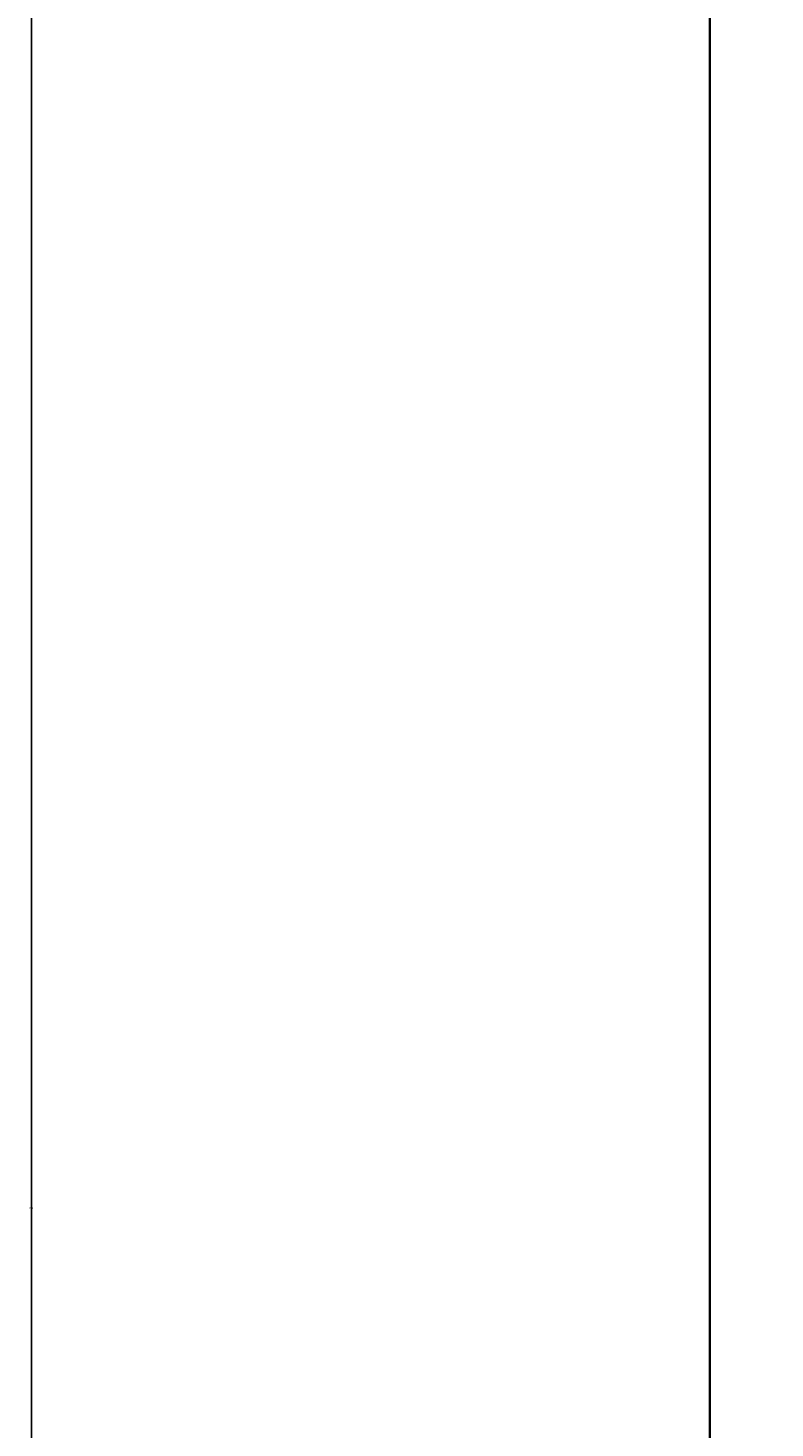
# Model space of a CAD drawing. Units: inches. Extents: x -61 to 1599, y -1316 to 257.
# Tile 96 of 204: x -61 to 22, y -166 to -10. Entities that reach past the tile are written whole.
import ezdxf

# ---------------------------------------------------------------- set-up
doc = ezdxf.new("R2010")
doc.units = ezdxf.units.IN
doc.header["$MEASUREMENT"] = 0
doc.layers.add('A-ANNO-DIMS', color=2, linetype='Continuous', lineweight=18)
doc.layers.add('WALLS', color=4, linetype='Continuous', lineweight=35)
doc.styles.get("Standard").update_dxf_attribs({"font": 'arial.ttf'})
doc.dimstyles.get("Standard").update_dxf_attribs({"dimtxt": 0.18, "dimasz": 0.18, "dimexe": 0.18, "dimexo": 0.0625, "dimgap": 0.09, "dimtad": 0, "dimtih": 1, "dimtoh": 1, "dimdec": 0, "dimzin": 0, "dimdsep": 46, "dimlunit": 3, "dimtxsty": 'Standard', "dimcen": 0.09, "dimadec": 0, "dimazin": 0, "dimtfac": 1, "dimtdec": 0, "dimtofl": 0, "dimtmove": 0, "dimatfit": 3, "dimfxl": 1, "dimtolj": 1, "dimtzin": 0, "dimarcsym": 0})

# ---------------------------------------------------------------- blocks, each defined once
blk = doc.blocks.new('*D687')
at = {"layer": 'A-ANNO-DIMS', "color": 0, "lineweight": -2, "transparency": 16777216}
for p, q in [((289.42, 181.68), (-61.08, 181.68)), ((-60.9, 181.5), (-60.9, -528.95)), ((-60.9, -1239.76), (-60.9, -529.32)), ((319.64, -1239.94), (-61.08, -1239.94))]:
    blk.add_line(p, q, dxfattribs=at)
at = {"layer": 'A-ANNO-DIMS', "color": 0, "transparency": 16777216}
for points in [[(-60.93, 181.5), (-60.87, 181.5), (-60.9, 181.68)], [(-60.93, -1239.76), (-60.87, -1239.76), (-60.9, -1239.94)]]:
    blk.add_solid(points, dxfattribs=at)
at = {"layer": 'DEFPOINTS', "color": 0, "transparency": 16777216}
for p in [(289.48, 181.68), (-60.9, -1239.94), (319.7, -1239.94)]:
    blk.add_point(p, dxfattribs=at)
at = {"layer": 'A-ANNO-DIMS', "color": 0, "transparency": 16777216, "insert": (-60.9, -529.13), "char_height": 0.18, "attachment_point": 5}
blk.add_mtext('\\A1;1421.6', dxfattribs=at)
blk = doc.blocks.new('*D691')
at = {"layer": 'A-ANNO-DIMS', "color": 0, "lineweight": -2, "transparency": 16777216}
for p, q in [((14.64, 157.68), (-61.08, 157.68)), ((-60.9, 157.5), (-60.9, -141.64)), ((-60.9, -441.14), (-60.9, -142)), ((14.64, -441.32), (-61.08, -441.32))]:
    blk.add_line(p, q, dxfattribs=at)
at = {"layer": 'A-ANNO-DIMS', "color": 0, "transparency": 16777216}
for points in [[(-60.93, 157.5), (-60.87, 157.5), (-60.9, 157.68)], [(-60.93, -441.14), (-60.87, -441.14), (-60.9, -441.32)]]:
    blk.add_solid(points, dxfattribs=at)
at = {"layer": 'DEFPOINTS', "color": 0, "transparency": 16777216}
for p in [(-60.9, 157.68), (14.7, 157.68), (14.7, -441.32)]:
    blk.add_point(p, dxfattribs=at)
at = {"layer": 'A-ANNO-DIMS', "color": 0, "transparency": 16777216, "insert": (-60.9, -141.82), "char_height": 0.18, "attachment_point": 5}
blk.add_mtext('\\A1;599', dxfattribs=at)
blk = doc.blocks.new('*D700')
at = {"layer": 'A-ANNO-DIMS', "color": 0, "lineweight": -2, "transparency": 16777216}
for p, q in [((14.7, -616.88), (14.7, 257.46)), ((179.75, -616.88), (179.75, 257.46)), ((14.88, 257.28), (96.77, 257.28)), ((179.57, 257.28), (97.68, 257.28))]:
    blk.add_line(p, q, dxfattribs=at)
at = {"layer": 'A-ANNO-DIMS', "color": 0, "transparency": 16777216}
for points in [[(14.88, 257.31), (14.88, 257.25), (14.7, 257.28)], [(179.57, 257.31), (179.57, 257.25), (179.75, 257.28)]]:
    blk.add_solid(points, dxfattribs=at)
at = {"layer": 'DEFPOINTS', "color": 0, "transparency": 16777216}
for p in [(179.75, 257.28), (14.7, -616.94), (179.75, -616.94)]:
    blk.add_point(p, dxfattribs=at)
at = {"layer": 'A-ANNO-DIMS', "color": 0, "transparency": 16777216, "insert": (97.23, 257.28), "char_height": 0.18, "attachment_point": 5}
blk.add_mtext('\\A1;165.05', dxfattribs=at)

msp = doc.modelspace()

# ---------------------------------------------------------------- linework, layer by layer
at = {"layer": 'WALLS'}
msp.add_line((14.7028, 157.6771), (14.7028, -441.3229), dxfattribs=at)

# ---------------------------------------------------------------- dimensions: what is measured, and where the dimension line sits
at = {"layer": 'A-ANNO-DIMS'}
dim = msp.add_linear_dim(base=(179.7521, 257.2771), p1=(14.7028, -616.9446), p2=(179.7521, -616.9446), dimstyle='Standard', override={"dimdec": 2, "dimlfac": 1, "dimrnd": 0, "dimzin": 0, "dimdsep": 46, "dimlunit": 2}, dxfattribs=at)
dim.commit()
dim.dimension.update_dxf_attribs({"geometry": '*D700', "text_midpoint": (97.2274, 257.2771)})
for base, p1, p2, override, picture, middle in [((-60.8972, -1239.9446), (289.4807, 181.6771), (319.7028, -1239.9446), {"dimdec": 1, "dimlfac": 1, "dimrnd": 0, "dimzin": 0, "dimdsep": 46, "dimlunit": 2}, '*D687', (-60.8972, -529.1337)), ((-60.8972, 157.6771), (14.7028, -441.3229), (14.7028, 157.6771), {"dimdec": 0, "dimlfac": 1, "dimrnd": 0, "dimzin": 0, "dimdsep": 46, "dimlunit": 2}, '*D691', (-60.8972, -141.8229))]:
    dim = msp.add_linear_dim(base=base, p1=p1, p2=p2, angle=90, dimstyle='Standard', override=override, dxfattribs=at)
    dim.commit()
    dim.dimension.update_dxf_attribs({"geometry": picture, "text_midpoint": middle})

doc.saveas('drawing.dxf')
